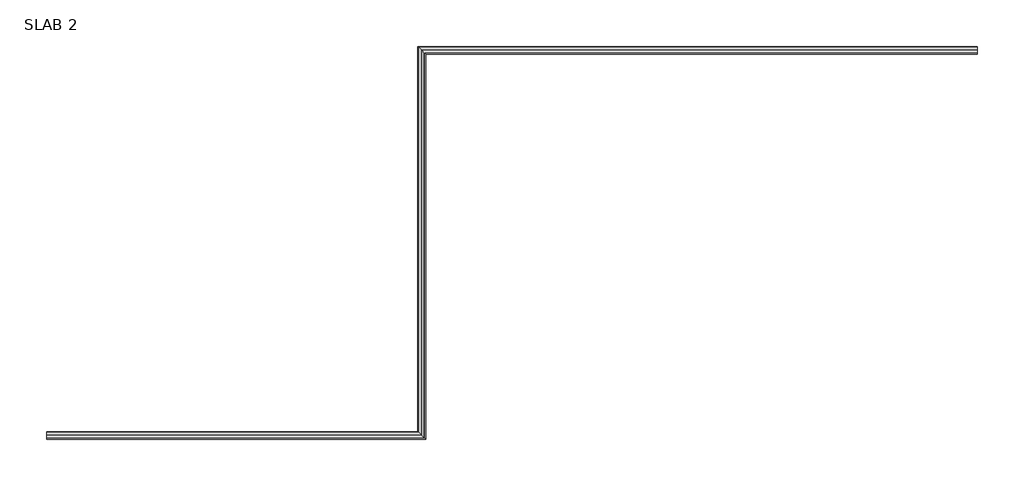
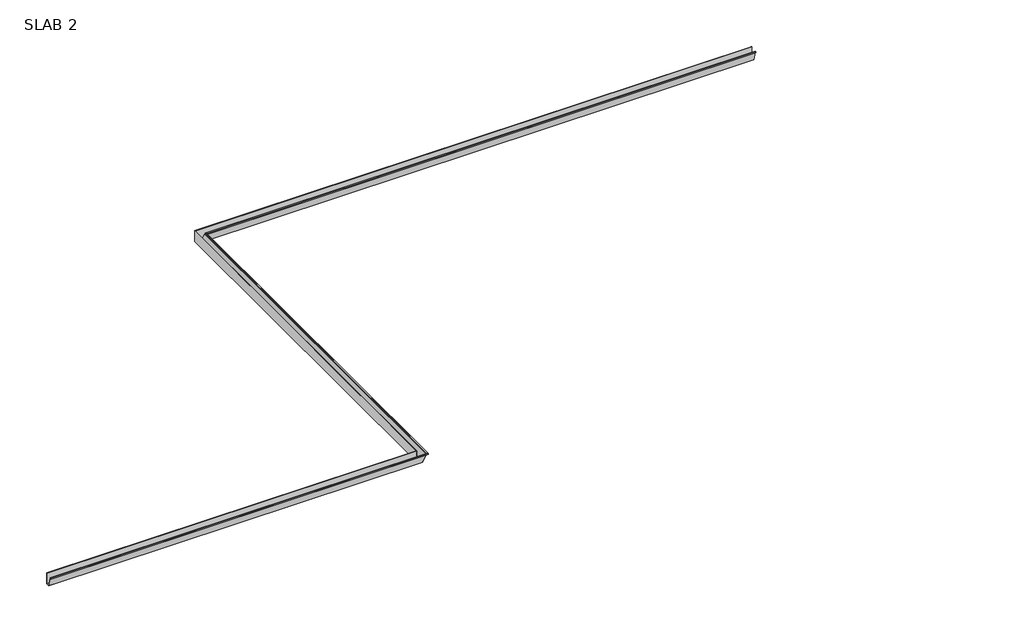
# One storey: 2 pipe segments.
"""IFC4 building model written with IfcOpenShell, lengths in millimetres."""

from ifc_helpers import new_model, si_unit, origin, place, context, project, spatial, faceted_brep, element, save

model = new_model("IFC4")

# Units and contexts
model_context = context("Model", 3, world=origin())
ifc_project = project(units=[si_unit("LENGTHUNIT", "METRE", prefix="MILLI")], contexts=[model_context])

# Site, building, storey
site = spatial("IfcSite", under=ifc_project)
building = spatial("IfcBuilding", under=site)
storey = spatial("IfcBuildingStorey", under=building, Name="SLAB 2", Elevation=7010.4)

# Pipe segments
placement = place(None, origin())
element("IfcPipeSegment", 1, ObjectType="Gutter - Bevel 5\" x 5\"", at=placement, inside=storey, context=model_context, shape_type="Brep", body=[
    faceted_brep([(-13154.5324866, 1409.0047421, 7772.4877675), (-13154.5324866, 1358.2047421, 7772.4877675), (-13154.5324866, 1320.1047421, 7899.4), (-13154.5324866, 1307.4047421, 7899.4), (-13154.5324866, 1307.4047421, 7912.1), (-13154.5324866, 1320.1047421, 7912.1), (-13154.5324866, 1320.1047421, 7908.925), (-13154.5324866, 1310.5797421, 7908.925), (-13154.5324866, 1310.5797421, 7902.575), (-13154.5324866, 1322.4670394, 7902.575), (-13154.5324866, 1360.5670394, 7775.6627675), (-13154.5324866, 1405.8297421, 7775.6627675), (-13154.5324866, 1405.8297421, 7924.8), (-13154.5324866, 1409.0047421, 7924.8), (-8223.6008651, 1409.0047421, 7772.4877675), (-8223.6008651, 1409.0047421, 7924.8), (-8220.4258651, 1405.8297421, 7924.8), (-8220.4258651, 1405.8297421, 7775.6627675), (-8175.1631624, 1360.5670394, 7775.6627675), (-8137.0631624, 1322.4670394, 7902.575), (-8125.1758651, 1310.5797421, 7902.575), (-8125.1758651, 1310.5797421, 7908.925), (-8134.7008651, 1320.1047421, 7908.925), (-8134.7008651, 1320.1047421, 7912.1), (-8122.0008651, 1307.4047421, 7912.1), (-8122.0008651, 1307.4047421, 7899.4), (-8134.7008651, 1320.1047421, 7899.4), (-8172.8008651, 1358.2047421, 7772.4877675)], [[[0, 1, 2, 3, 4, 5, 6, 7, 8, 9, 10, 11, 12, 13]], [[14, 15, 16, 17, 18, 19, 20, 21, 22, 23, 24, 25, 26, 27]], [[1, 0, 14, 27]], [[2, 1, 27, 26]], [[3, 2, 26, 25]], [[4, 3, 25, 24]], [[5, 4, 24, 23]], [[6, 5, 23, 22]], [[7, 6, 22, 21]], [[8, 7, 21, 20]], [[9, 8, 20, 19]], [[10, 9, 19, 18]], [[11, 10, 18, 17]], [[12, 11, 17, 16]], [[13, 12, 16, 15]], [[0, 13, 15, 14]]]),
])
element("IfcPipeSegment", 2, ObjectType="Gutter - Bevel 5\" x 5\"", at=placement, inside=storey, context=model_context, shape_type="Brep", body=[
    faceted_brep([(-8223.6008651, 1409.0047421, 7772.4877675), (-8172.8008651, 1358.2047421, 7772.4877675), (-8134.7008651, 1320.1047421, 7899.4), (-8122.0008651, 1307.4047421, 7899.4), (-8122.0008651, 1307.4047421, 7912.1), (-8134.7008651, 1320.1047421, 7912.1), (-8134.7008651, 1320.1047421, 7908.925), (-8125.1758651, 1310.5797421, 7908.925), (-8125.1758651, 1310.5797421, 7902.575), (-8137.0631624, 1322.4670394, 7902.575), (-8175.1631624, 1360.5670394, 7775.6627675), (-8220.4258651, 1405.8297421, 7775.6627675), (-8220.4258651, 1405.8297421, 7924.8), (-8223.6008651, 1409.0047421, 7924.8), (-8223.6008651, 6527.1047421, 7772.4877675), (-8172.8008651, 6476.3047421, 7772.4877675), (-8134.7008651, 6438.2047421, 7899.4), (-8122.0008651, 6425.5047421, 7899.4), (-8122.0008651, 6425.5047421, 7912.1), (-8134.7008651, 6438.2047421, 7912.1), (-8134.7008651, 6438.2047421, 7908.925), (-8125.1758651, 6428.6797421, 7908.925), (-8125.1758651, 6428.6797421, 7902.575), (-8137.0631624, 6440.5670394, 7902.575), (-8175.1631624, 6478.6670394, 7775.6627675), (-8220.4258651, 6523.9297421, 7775.6627675), (-8220.4258651, 6523.9297421, 7924.8), (-8223.6008651, 6527.1047421, 7924.8), (-794.1008651, 6527.1047421, 7772.4877675), (-794.1008651, 6527.1047421, 7924.8), (-794.1008651, 6523.9297421, 7924.8), (-794.1008651, 6523.9297421, 7775.6627675), (-794.1008651, 6478.6670394, 7775.6627675), (-794.1008651, 6440.5670394, 7902.575), (-794.1008651, 6428.6797421, 7902.575), (-794.1008651, 6428.6797421, 7908.925), (-794.1008651, 6438.2047421, 7908.925), (-794.1008651, 6438.2047421, 7912.1), (-794.1008651, 6425.5047421, 7912.1), (-794.1008651, 6425.5047421, 7899.4), (-794.1008651, 6438.2047421, 7899.4), (-794.1008651, 6476.3047421, 7772.4877675)], [[[0, 1, 2, 3, 4, 5, 6, 7, 8, 9, 10, 11, 12, 13]], [[1, 0, 14, 15]], [[2, 1, 15, 16]], [[3, 2, 16, 17]], [[4, 3, 17, 18]], [[5, 4, 18, 19]], [[6, 5, 19, 20]], [[7, 6, 20, 21]], [[8, 7, 21, 22]], [[9, 8, 22, 23]], [[10, 9, 23, 24]], [[11, 10, 24, 25]], [[12, 11, 25, 26]], [[13, 12, 26, 27]], [[0, 13, 27, 14]], [[28, 29, 30, 31, 32, 33, 34, 35, 36, 37, 38, 39, 40, 41]], [[15, 14, 28, 41]], [[16, 15, 41, 40]], [[17, 16, 40, 39]], [[18, 17, 39, 38]], [[19, 18, 38, 37]], [[20, 19, 37, 36]], [[21, 20, 36, 35]], [[22, 21, 35, 34]], [[23, 22, 34, 33]], [[24, 23, 33, 32]], [[25, 24, 32, 31]], [[26, 25, 31, 30]], [[27, 26, 30, 29]], [[14, 27, 29, 28]]]),
])

save(model, "model.ifc")

# Revit data of these elements
# Elements 1, 2 (IfcPipeSegment, "Gutter - Bevel 5\" x 5\"")
#   Phase Created = New Construction
#   Materials on its faces: "Default Roof"
# Materials
#   "Default Roof": colour RGB 88 101 114, transparency 0
